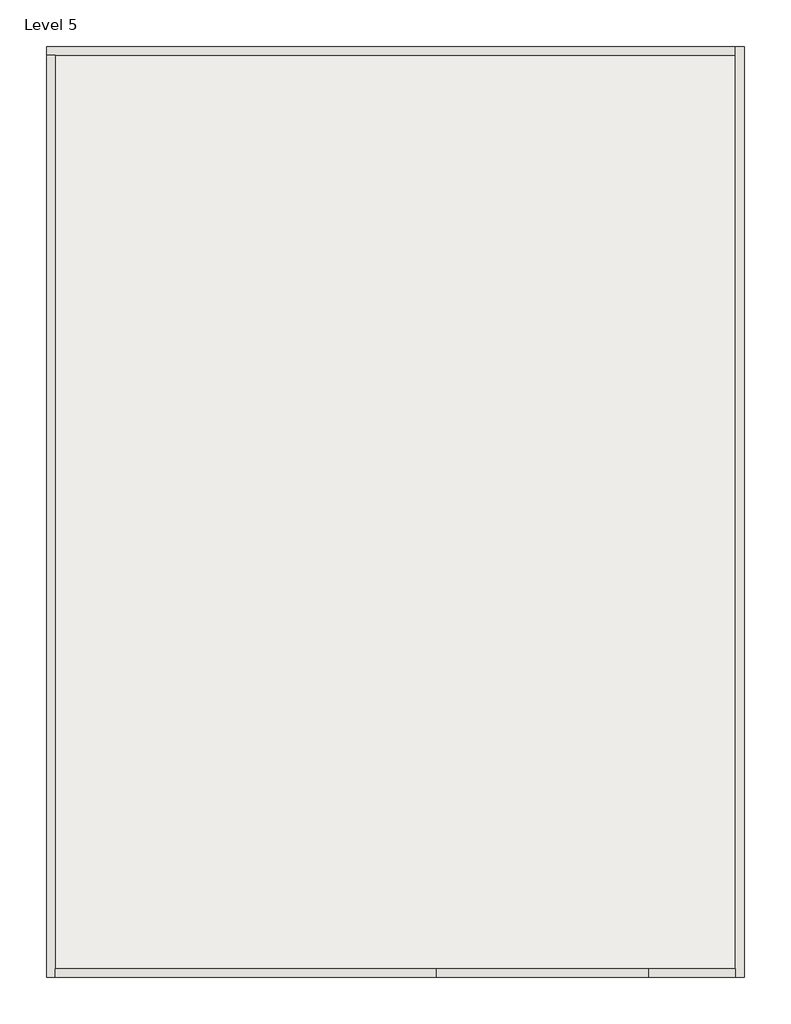
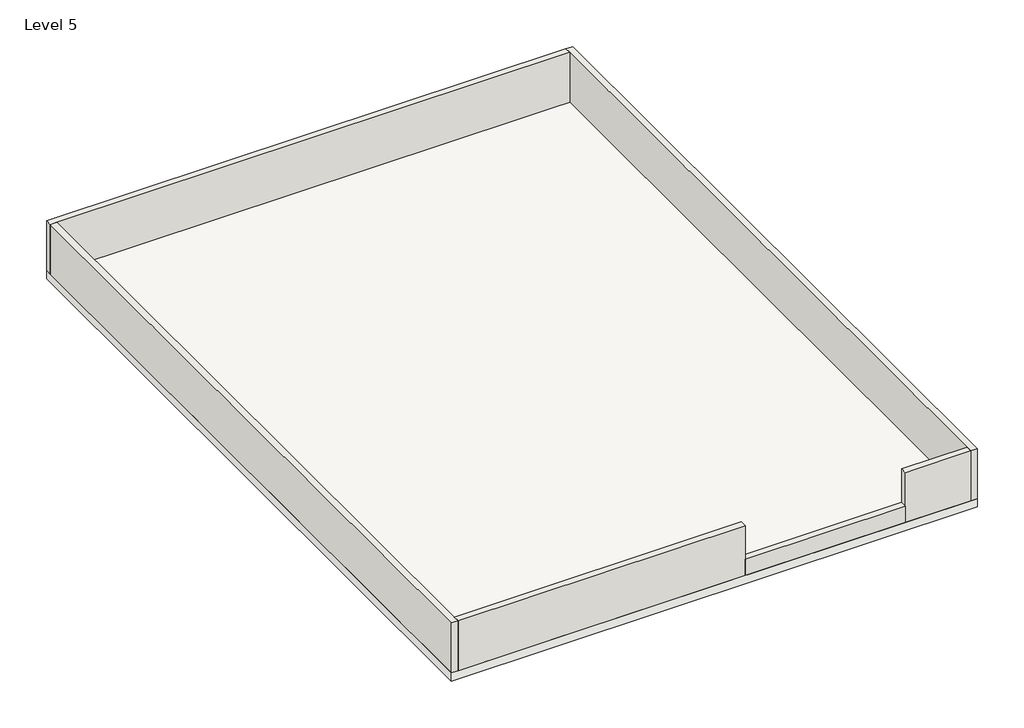
# One storey: 6 walls, 1 slab.
"""IFC4 building model written with IfcOpenShell, lengths in millimetres."""

from ifc_helpers import new_model, si_unit, frame, origin, place, context, project, spatial, polyline, outline, extrude, faceted_brep, element, save

model = new_model("IFC4")

# Units and contexts
model_context = context("Model", 3, world=origin())
ifc_project = project(units=[si_unit("LENGTHUNIT", "METRE", prefix="MILLI")], contexts=[model_context])

# Site, building, storey
site = spatial("IfcSite", under=ifc_project)
building = spatial("IfcBuilding", under=site)
storey = spatial("IfcBuildingStorey", under=building, Name="Level 5", Elevation=6400.8)

# Slab
placement = place(None, origin())
element("IfcSlab", 1, ObjectType="6\" floor", at=placement, inside=storey, context=model_context, shape_type="SweptSolid", body=[
    extrude(outline(polyline([(-4410.3551496, 10306.002641), (-4410.3551496, -1885.997359), (-13554.3551496, -1885.997359), (-13554.3551496, 10306.002641), (-4410.3551496, 10306.002641)])), frame((0.0, 0.0, 6248.4), z_axis=(0.0, 0.0, 1.0), x_axis=(1.0, 0.0, 0.0)), (0.0, 0.0, 1.0), 152.4),
])

# Walls
element("IfcWall", 2, ObjectType="4.5\" INNER WALL", at=placement, inside=storey, context=model_context, shape_type="Brep", body=[
    faceted_brep([(-13554.3551496, 10191.702641, 6400.8), (-13440.0551496, 10191.702641, 6400.8), (-4524.6551496, 10191.702641, 6400.8), (-4524.6551496, 10191.702641, 7315.2), (-13440.0551496, 10191.702641, 7315.2), (-13554.3551496, 10191.702641, 7315.2), (-13554.3551496, 10306.002641, 6400.8), (-13554.3551496, 10306.002641, 7315.2), (-4524.6551496, 10306.002641, 7315.2), (-4524.6551496, 10306.002641, 6400.8)], [[[0, 1, 2, 3, 4, 5]], [[6, 7, 8, 9]], [[2, 1, 0, 6, 9]], [[5, 4, 3, 8, 7]], [[0, 5, 7, 6]], [[3, 2, 9, 8]]]),
])
element("IfcWall", 3, ObjectType="4.5\" INNER WALL", at=placement, inside=storey, context=model_context, shape_type="Brep", body=[
    faceted_brep([(-13440.0551496, -1885.997359, 6400.8), (-13440.0551496, -1771.697359, 6400.8), (-13440.0551496, 10191.702641, 6400.8), (-13440.0551496, 10191.702641, 7315.2), (-13440.0551496, -1771.697359, 7315.2), (-13440.0551496, -1885.997359, 7315.2), (-13554.3551496, -1885.997359, 6400.8), (-13554.3551496, -1885.997359, 7315.2), (-13554.3551496, 10191.702641, 7315.2), (-13554.3551496, 10191.702641, 6400.8)], [[[0, 1, 2, 3, 4, 5]], [[6, 7, 8, 9]], [[2, 1, 0, 6, 9]], [[5, 4, 3, 8, 7]], [[0, 5, 7, 6]], [[3, 2, 9, 8]]]),
])
element("IfcWall", 4, ObjectType="4.5\" INNER WALL", at=placement, inside=storey, context=model_context, shape_type="Brep", body=[
    faceted_brep([(-8448.9551496, -1771.697359, 6400.8), (-13440.0551496, -1771.697359, 6400.8), (-13440.0551496, -1771.697359, 7315.2), (-8448.9551496, -1771.697359, 7315.2), (-8448.9551496, -1771.697359, 6698.4419146), (-8448.9551496, -1885.997359, 6400.8), (-8448.9551496, -1885.997359, 6698.4419146), (-8448.9551496, -1885.997359, 7315.2), (-13440.0551496, -1885.997359, 7315.2), (-13440.0551496, -1885.997359, 6400.8)], [[[0, 1, 2, 3, 4]], [[5, 6, 7, 8, 9]], [[1, 0, 5, 9]], [[3, 2, 8, 7]], [[0, 4, 3, 7, 6, 5]], [[2, 1, 9, 8]]]),
])
element("IfcWall", 5, ObjectType="4.5\" INNER WALL", at=placement, inside=storey, context=model_context, shape_type="Brep", body=[
    faceted_brep([(-4524.6551496, 10306.002641, 6400.8), (-4524.6551496, 10191.702641, 6400.8), (-4524.6551496, -1771.697359, 6400.8), (-4524.6551496, -1885.997359, 6400.8), (-4524.6551496, -1885.997359, 7315.2), (-4524.6551496, -1771.697359, 7315.2), (-4524.6551496, 10191.702641, 7315.2), (-4524.6551496, 10306.002641, 7315.2), (-4410.3551496, 10306.002641, 6400.8), (-4410.3551496, 10306.002641, 7315.2), (-4410.3551496, -1885.997359, 7315.2), (-4410.3551496, -1885.997359, 6400.8)], [[[0, 1, 2, 3, 4, 5, 6, 7]], [[8, 9, 10, 11]], [[3, 2, 1, 0, 8, 11]], [[7, 6, 5, 4, 10, 9]], [[0, 7, 9, 8]], [[4, 3, 11, 10]]]),
])
element("IfcWall", 6, ObjectType="4.5\" INNER WALL", at=placement, inside=storey, context=model_context, shape_type="SweptSolid", body=[
    extrude(outline(polyline([(-5661.3051496, -1885.997359), (-8448.9551496, -1885.997359), (-8448.9551496, -1771.697359), (-5661.3051496, -1771.697359), (-5661.3051496, -1885.997359)])), frame((0.0, 0.0, 6400.8), z_axis=(0.0, 0.0, 1.0), x_axis=(1.0, 0.0, 0.0)), (0.0, 0.0, 1.0), 297.6419146),
])
element("IfcWall", 7, ObjectType="4.5\" INNER WALL", at=placement, inside=storey, context=model_context, shape_type="Brep", body=[
    faceted_brep([(-5661.3051496, -1885.997359, 6400.8), (-4524.6551496, -1885.997359, 6400.8), (-4524.6551496, -1885.997359, 7315.2), (-5661.3051496, -1885.997359, 7315.2), (-5661.3051496, -1885.997359, 6698.4419146), (-5661.3051496, -1771.697359, 6400.8), (-5661.3051496, -1771.697359, 6698.4419146), (-5661.3051496, -1771.697359, 7315.2), (-4524.6551496, -1771.697359, 7315.2), (-4524.6551496, -1771.697359, 6400.8)], [[[0, 1, 2, 3, 4]], [[5, 6, 7, 8, 9]], [[1, 0, 5, 9]], [[3, 2, 8, 7]], [[0, 4, 3, 7, 6, 5]], [[2, 1, 9, 8]]]),
])

save(model, "model.ifc")

# Revit data of these elements
# Type "6\" floor"
#   Assembly Code = "B1010"
#   Function = 0
#   Layers, outside or top first: 0' - 6" no material (function 1)
# Type "4.5\" INNER WALL"
#   Assembly Code = "B2010"
#   Layers, outside or top first: 0' - 4 1/2" "Damp-proofing" (function 1)
# Element 1 (IfcSlab, "6\" floor")
#   Height Offset From Level = 0' - 0"
#   Phase Created = New Construction
#   Materials on its faces: "Default Floor"
# Elements 2, 3, 4, 5, 7 (IfcWall, "4.5\" INNER WALL")
#   Top Offset = 0' - 0"
#   Base Offset = 0' - 0"
#   wall height = 3' - 0"
#   Phase Created = New Construction
#   Base Constraint = Level 5
#   Top Constraint = Level 6
#   Materials on its faces: "Damp-proofing"
# Element 6 (IfcWall, "4.5\" INNER WALL")
#   Top Offset = -2' - 0.28181"
#   Base Offset = 0' - 0"
#   wall height = 0' - 11.71819"
#   Phase Created = New Construction
#   Base Constraint = Level 5
#   Top Constraint = Level 6
#   Materials on its faces: "Damp-proofing"
# Materials
#   "Damp-proofing": class "Generic", colour RGB 127 127 127, transparency 0, Description = "Damp-proofing", Cost = 0
#   "Default Floor": colour RGB 128 128 128, transparency 0, Cost = 0
